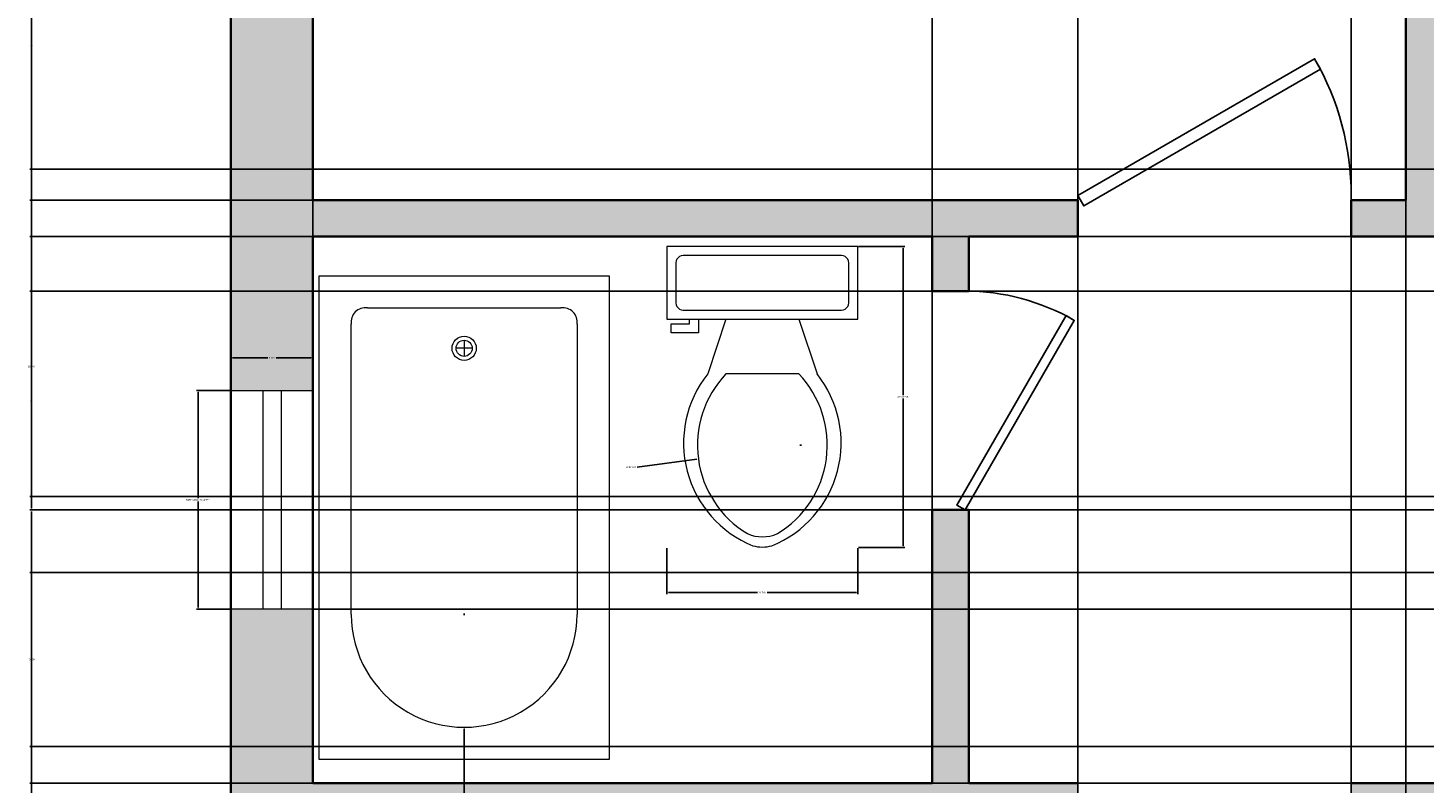
# Model space of a CAD drawing. Units: inches. Extents: x 2800 to 3283, y 1752 to 2114.
# Tile 2 of 6: x 2800 to 2954, y 1903 to 1986. Entities that reach past the tile are written whole.
import ezdxf

# ---------------------------------------------------------------- set-up
doc = ezdxf.new("R2010")
doc.units = ezdxf.units.IN
for name, color, linetype, lineweight in [('A-ANNO-DIMS', 2, 'Continuous', 18), ('A-DOOR', 3, 'Continuous', 25), ('A-FLOR-FIXT', 9, 'Continuous', 18), ('A-GLAZ', 4, 'Continuous', 18), ('A-WALL', 7, 'Continuous', 35)]:
    doc.layers.add(name, color=color, linetype=linetype, lineweight=lineweight)
doc.layers.add('A-WALL-PATT', color=18, linetype='Continuous', lineweight=13, true_color=0x000000)
doc.styles.get("Standard").update_dxf_attribs({"font": 'arial.ttf'})
doc.dimstyles.get("Standard").update_dxf_attribs({"dimtxt": 0.18, "dimasz": 0.18, "dimexe": 0.18, "dimexo": 0.0625, "dimgap": 0.09, "dimtad": 0, "dimtih": 1, "dimtoh": 1, "dimdec": 4, "dimzin": 0, "dimdsep": 46, "dimtxsty": 'Standard', "dimcen": 0.09, "dimadec": 0, "dimazin": 0, "dimtfac": 1, "dimtdec": 4, "dimtofl": 0, "dimtmove": 0, "dimatfit": 3, "dimfxl": 1, "dimtolj": 1, "dimtzin": 0, "dimarcsym": 0})

# ---------------------------------------------------------------- blocks, each defined once
blk = doc.blocks.new('Bath Tub - 26 x 60 in.')
for p, q in [((9, -17), (9, -19)), ((8, -18), (10, -18))]:
    blk.add_line(p, q)
blk.add_lwpolyline([(0, -36), (0, 0), (60, 0), (60, -36)], close=True)
for points in [[(6, -4), (42, -4)], [(4, -30), (4, -6)], [(42, -32), (6, -32)]]:
    blk.add_lwpolyline(points)
for radius in [1.5, 1]:
    blk.add_circle((9, -18), radius)
for centre, radius, start, end in [((5.75, -5.75), 1.77, 81.8699, 188.1301), ((42, -18), 14, 270, 90), ((5.75, -30.25), 1.77, 171.8699, 278.1301)]:
    blk.add_arc(centre, radius, start, end)
blk = doc.blocks.new('Toilet - top')
for p, q in [((9.5, -6), (9.5, -2)), ((-10, -8.5), (-8, -8.5)), ((-10, -9.5), (-10, -8.5)), ((-8, -8.5), (-8, -8)), ((-7, -8), (-7, -9.5)), ((-4, -8), (-6, -14)), ((4, -8), (6, -14)), ((-7, -9.5), (-10, -9.5)), ((4, -14), (-4, -14))]:
    blk.add_line(p, q)
blk.add_lwpolyline([(10.5, -8), (10.5, 0), (-10.5, 0), (-10.5, -8)], close=True)
for points in [[(8.5, -1), (-8.5, -1)], [(-9.5, -2), (-9.5, -6)], [(-8.5, -7), (8.5, -7)]]:
    blk.add_lwpolyline(points)
for centre, radius, start, end in [((-8.62, -1.88), 0.884, 81.8699, 188.1301), ((8.62, -1.88), 0.884, 351.8699, 98.1301), ((-8.62, -6.12), 0.884, 171.8699, 278.1301), ((8.62, -6.12), 0.884, 261.8699, 8.1301), ((3.52, -21.58), 12.17, 141.4691, 247.9714), ((4.2, -21.82), 11.33, 136.3677, 238.9468), ((-3.52, -21.58), 12.17, 292.0284, 38.5307), ((-4.2, -21.82), 11.33, 301.053, 43.6321), ((0, -27.88), 4, 245.7318, 294.2682), ((0, -29), 4, 254.8605, 285.1395)]:
    blk.add_arc(centre, radius, start, end)
blk = doc.blocks.new('*U12')
for p, q in [((0, 0), (0, -6)), ((40, 0), (40, -6))]:
    blk.add_line(p, q)
blk.add_lwpolyline([(0, 0), (34.64, 20), (35.52, 18.48), (0.87, -1.52)], close=True)
blk.add_arc((0, 0), 40, 0, 30)
blk = doc.blocks.new('WIN-24')
for p, q in [((3.5, 24), (3.5, 0)), ((5.5, 24), (5.5, 0))]:
    blk.add_line(p, q)
for points in [[(0, 24), (9, 24)], [(9, 0), (0, 0)]]:
    blk.add_lwpolyline(points)
blk = doc.blocks.new('*D21')
at = {"layer": 'A-ANNO-DIMS', "color": 0, "lineweight": -2, "transparency": 16777216}
for p, q in [((2822.48, 1946.35), (2818.76, 1946.35)), ((2818.94, 1946.17), (2818.94, 1934.54)), ((2818.94, 1922.53), (2818.94, 1934.17)), ((2822.48, 1922.35), (2818.76, 1922.35))]:
    blk.add_line(p, q, dxfattribs=at)
at = {"layer": 'A-ANNO-DIMS', "color": 0, "transparency": 16777216}
for points in [[(2818.91, 1946.17), (2818.97, 1946.17), (2818.94, 1946.35)], [(2818.91, 1922.53), (2818.97, 1922.53), (2818.94, 1922.35)]]:
    blk.add_solid(points, dxfattribs=at)
at = {"layer": 'Defpoints', "color": 0, "transparency": 16777216}
for p in [(2818.94, 1946.35), (2822.54, 1946.35), (2822.54, 1922.35)]:
    blk.add_point(p, dxfattribs=at)
at = {"layer": 'A-ANNO-DIMS', "color": 0, "transparency": 16777216, "insert": (2818.94, 1934.35), "char_height": 0.18, "attachment_point": 5}
blk.add_mtext('\\A1;BATH WINDOW 24 TYP.', dxfattribs=at)
blk = doc.blocks.new('*D22')
at = {"layer": 'A-ANNO-DIMS', "color": 0, "lineweight": -2, "transparency": 16777216}
for p, q in [((2822.54, 1946.42), (2822.54, 1950.13)), ((2822.72, 1949.95), (2826.59, 1949.95)), ((2831.36, 1949.95), (2827.5, 1949.95)), ((2831.54, 1946.42), (2831.54, 1950.13))]:
    blk.add_line(p, q, dxfattribs=at)
at = {"layer": 'A-ANNO-DIMS', "color": 0, "transparency": 16777216}
for points in [[(2822.72, 1949.98), (2822.72, 1949.92), (2822.54, 1949.95)], [(2831.36, 1949.98), (2831.36, 1949.92), (2831.54, 1949.95)]]:
    blk.add_solid(points, dxfattribs=at)
at = {"layer": 'Defpoints', "color": 0, "transparency": 16777216}
for p in [(2831.54, 1949.95), (2822.54, 1946.35), (2831.54, 1946.35)]:
    blk.add_point(p, dxfattribs=at)
at = {"layer": 'A-ANNO-DIMS', "color": 0, "transparency": 16777216, "insert": (2827.04, 1949.95), "char_height": 0.18, "attachment_point": 5}
blk.add_mtext('\\A1;9 TYP.', dxfattribs=at)
blk = doc.blocks.new('*D33')
at = {"layer": 'A-ANNO-DIMS', "color": 0, "lineweight": -2, "transparency": 16777216}
for p, q in [((2891.45, 1962.18), (2896.53, 1962.18)), ((2896.35, 1962), (2896.35, 1945.84)), ((2896.35, 1929.31), (2896.35, 1945.47)), ((2891.45, 1929.13), (2896.53, 1929.13))]:
    blk.add_line(p, q, dxfattribs=at)
at = {"layer": 'A-ANNO-DIMS', "color": 0, "transparency": 16777216}
for points in [[(2896.32, 1962), (2896.38, 1962), (2896.35, 1962.18)], [(2896.32, 1929.31), (2896.38, 1929.31), (2896.35, 1929.13)]]:
    blk.add_solid(points, dxfattribs=at)
at = {"layer": 'Defpoints', "color": 0, "transparency": 16777216}
for p in [(2891.39, 1962.18), (2896.35, 1962.18), (2891.39, 1929.13)]:
    blk.add_point(p, dxfattribs=at)
at = {"layer": 'A-ANNO-DIMS', "color": 0, "transparency": 16777216, "insert": (2896.35, 1945.66), "char_height": 0.18, "attachment_point": 5}
blk.add_mtext('\\A1;WC 33 TYP.', dxfattribs=at)
blk = doc.blocks.new('*D34')
at = {"layer": 'A-ANNO-DIMS', "color": 0, "lineweight": -2, "transparency": 16777216}
for p, q in [((2870.39, 1929.07), (2870.39, 1924)), ((2891.39, 1929.07), (2891.39, 1924)), ((2870.57, 1924.18), (2880.36, 1924.18)), ((2891.21, 1924.18), (2881.42, 1924.18))]:
    blk.add_line(p, q, dxfattribs=at)
at = {"layer": 'A-ANNO-DIMS', "color": 0, "transparency": 16777216}
for points in [[(2870.57, 1924.21), (2870.57, 1924.15), (2870.39, 1924.18)], [(2891.21, 1924.21), (2891.21, 1924.15), (2891.39, 1924.18)]]:
    blk.add_solid(points, dxfattribs=at)
at = {"layer": 'Defpoints', "color": 0, "transparency": 16777216}
for p in [(2870.39, 1929.13), (2891.39, 1929.13), (2891.39, 1924.18)]:
    blk.add_point(p, dxfattribs=at)
at = {"layer": 'A-ANNO-DIMS', "color": 0, "transparency": 16777216, "insert": (2880.89, 1924.18), "char_height": 0.18, "attachment_point": 5}
blk.add_mtext('\\A1;21 TYP.', dxfattribs=at)
blk = doc.blocks.new('*D44')
at = {"layer": 'A-ANNO-DIMS', "color": 0, "lineweight": -2, "transparency": 16777216}
for p, q in [((2822.48, 2092.27), (2800.45, 2092.27)), ((2800.63, 2092.09), (2800.63, 1933.45)), ((2800.63, 1774.45), (2800.63, 1933.09)), ((2822.48, 1774.27), (2800.45, 1774.27))]:
    blk.add_line(p, q, dxfattribs=at)
at = {"layer": 'A-ANNO-DIMS', "color": 0, "transparency": 16777216}
for points in [[(2800.6, 2092.09), (2800.66, 2092.09), (2800.63, 2092.27)], [(2800.6, 1774.45), (2800.66, 1774.45), (2800.63, 1774.27)]]:
    blk.add_solid(points, dxfattribs=at)
at = {"layer": 'Defpoints', "color": 0, "transparency": 16777216}
for p in [(2800.63, 2092.27), (2822.54, 2092.27), (2822.54, 1774.27)]:
    blk.add_point(p, dxfattribs=at)
at = {"layer": 'A-ANNO-DIMS', "color": 0, "transparency": 16777216, "insert": (2800.63, 1933.27), "char_height": 0.18, "attachment_point": 5}
blk.add_mtext('\\A1;318', dxfattribs=at)
blk = doc.blocks.new('*D45')
at = {"layer": 'A-ANNO-DIMS', "color": 0, "lineweight": -2, "transparency": 16777216}
for p, q in [((2831.54, 1967.33), (2831.54, 2114.36)), ((2831.72, 2114.18), (2891.26, 2114.18)), ((2951.36, 2114.18), (2891.82, 2114.18)), ((2951.54, 1967.33), (2951.54, 2114.36))]:
    blk.add_line(p, q, dxfattribs=at)
at = {"layer": 'A-ANNO-DIMS', "color": 0, "transparency": 16777216}
for points in [[(2831.72, 2114.21), (2831.72, 2114.15), (2831.54, 2114.18)], [(2951.36, 2114.21), (2951.36, 2114.15), (2951.54, 2114.18)]]:
    blk.add_solid(points, dxfattribs=at)
at = {"layer": 'Defpoints', "color": 0, "transparency": 16777216}
for p in [(2951.54, 2114.18), (2831.54, 1967.27), (2951.54, 1967.27)]:
    blk.add_point(p, dxfattribs=at)
at = {"layer": 'A-ANNO-DIMS', "color": 0, "transparency": 16777216, "insert": (2891.54, 2114.18), "char_height": 0.18, "attachment_point": 5}
blk.add_mtext('\\A1;120', dxfattribs=at)
blk = doc.blocks.new('*D49')
at = {"layer": 'A-ANNO-DIMS', "color": 0, "lineweight": -2, "transparency": 16777216}
for p, q in [((2831.48, 2083.27), (2800.45, 2083.27)), ((2800.63, 2083.09), (2800.63, 2025.45)), ((2800.63, 1967.45), (2800.63, 2025.09)), ((2831.48, 1967.27), (2800.45, 1967.27))]:
    blk.add_line(p, q, dxfattribs=at)
at = {"layer": 'A-ANNO-DIMS', "color": 0, "transparency": 16777216}
for points in [[(2800.6, 2083.09), (2800.66, 2083.09), (2800.63, 2083.27)], [(2800.6, 1967.45), (2800.66, 1967.45), (2800.63, 1967.27)]]:
    blk.add_solid(points, dxfattribs=at)
at = {"layer": 'Defpoints', "color": 0, "transparency": 16777216}
for p in [(2800.63, 2083.27), (2831.54, 2083.27), (2831.54, 1967.27)]:
    blk.add_point(p, dxfattribs=at)
at = {"layer": 'A-ANNO-DIMS', "color": 0, "transparency": 16777216, "insert": (2800.63, 2025.27), "char_height": 0.18, "attachment_point": 5}
blk.add_mtext('\\A1;116', dxfattribs=at)
blk = doc.blocks.new('*D50')
at = {"layer": 'A-ANNO-DIMS', "color": 0, "lineweight": -2, "transparency": 16777216}
for p, q in [((2831.48, 1963.27), (2800.45, 1963.27)), ((2800.63, 1963.09), (2800.63, 1933.45)), ((2800.63, 1903.45), (2800.63, 1933.09)), ((2831.48, 1903.27), (2800.45, 1903.27))]:
    blk.add_line(p, q, dxfattribs=at)
at = {"layer": 'A-ANNO-DIMS', "color": 0, "transparency": 16777216}
for points in [[(2800.6, 1963.09), (2800.66, 1963.09), (2800.63, 1963.27)], [(2800.6, 1903.45), (2800.66, 1903.45), (2800.63, 1903.27)]]:
    blk.add_solid(points, dxfattribs=at)
at = {"layer": 'Defpoints', "color": 0, "transparency": 16777216}
for p in [(2800.63, 1963.27), (2831.54, 1963.27), (2831.54, 1903.27)]:
    blk.add_point(p, dxfattribs=at)
at = {"layer": 'A-ANNO-DIMS', "color": 0, "transparency": 16777216, "insert": (2800.63, 1933.27), "char_height": 0.18, "attachment_point": 5}
blk.add_mtext('\\A1;60', dxfattribs=at)
blk = doc.blocks.new('*D54')
at = {"layer": 'A-ANNO-DIMS', "color": 0, "lineweight": -2, "transparency": 16777216}
for p, q in [((2831.54, 1903.33), (2831.54, 2114.36)), ((2831.72, 2114.18), (2865.32, 2114.18)), ((2899.36, 2114.18), (2865.76, 2114.18)), ((2899.54, 1903.33), (2899.54, 2114.36))]:
    blk.add_line(p, q, dxfattribs=at)
at = {"layer": 'A-ANNO-DIMS', "color": 0, "transparency": 16777216}
for points in [[(2831.72, 2114.21), (2831.72, 2114.15), (2831.54, 2114.18)], [(2899.36, 2114.21), (2899.36, 2114.15), (2899.54, 2114.18)]]:
    blk.add_solid(points, dxfattribs=at)
at = {"layer": 'Defpoints', "color": 0, "transparency": 16777216}
for p in [(2899.54, 2114.18), (2831.54, 1903.27), (2899.54, 1903.27)]:
    blk.add_point(p, dxfattribs=at)
at = {"layer": 'A-ANNO-DIMS', "color": 0, "transparency": 16777216, "insert": (2865.54, 2114.18), "char_height": 0.18, "attachment_point": 5}
blk.add_mtext('\\A1;68', dxfattribs=at)
blk = doc.blocks.new('*D64')
at = {"layer": 'A-ANNO-DIMS', "color": 0, "lineweight": -2, "transparency": 16777216}
for p, q in [((2831.61, 1922.35), (3282.64, 1922.35)), ((3282.46, 1922.17), (3282.46, 1912.99)), ((3282.46, 1903.45), (3282.46, 1912.63)), ((2831.61, 1903.27), (3282.64, 1903.27))]:
    blk.add_line(p, q, dxfattribs=at)
at = {"layer": 'A-ANNO-DIMS', "color": 0, "transparency": 16777216}
for points in [[(3282.43, 1922.17), (3282.49, 1922.17), (3282.46, 1922.35)], [(3282.43, 1903.45), (3282.49, 1903.45), (3282.46, 1903.27)]]:
    blk.add_solid(points, dxfattribs=at)
at = {"layer": 'Defpoints', "color": 0, "transparency": 16777216}
for p in [(2831.54, 1922.35), (3282.46, 1922.35), (2831.54, 1903.27)]:
    blk.add_point(p, dxfattribs=at)
at = {"layer": 'A-ANNO-DIMS', "color": 0, "transparency": 16777216, "insert": (3282.46, 1912.81), "char_height": 0.18, "attachment_point": 5}
blk.add_mtext('\\A1;19.085', dxfattribs=at)
blk = doc.blocks.new('*D65')
at = {"layer": 'A-ANNO-DIMS', "color": 0, "lineweight": -2, "transparency": 16777216}
for p, q in [((3251.48, 1926.4), (2800.45, 1926.4)), ((2800.63, 1926.22), (2800.63, 1917.02)), ((2800.63, 1907.45), (2800.63, 1916.65)), ((3251.48, 1907.27), (2800.45, 1907.27))]:
    blk.add_line(p, q, dxfattribs=at)
at = {"layer": 'A-ANNO-DIMS', "color": 0, "transparency": 16777216}
for points in [[(2800.6, 1926.22), (2800.66, 1926.22), (2800.63, 1926.4)], [(2800.6, 1907.45), (2800.66, 1907.45), (2800.63, 1907.27)]]:
    blk.add_solid(points, dxfattribs=at)
at = {"layer": 'Defpoints', "color": 0, "transparency": 16777216}
for p in [(2800.63, 1926.4), (3251.54, 1926.4), (3251.54, 1907.27)]:
    blk.add_point(p, dxfattribs=at)
at = {"layer": 'A-ANNO-DIMS', "color": 0, "transparency": 16777216, "insert": (2800.63, 1916.83), "char_height": 0.18, "attachment_point": 5}
blk.add_mtext('\\A1;19.128', dxfattribs=at)
blk = doc.blocks.new('*D66')
at = {"layer": 'A-ANNO-DIMS', "color": 0, "lineweight": -2, "transparency": 16777216}
for p, q in [((2915.54, 1899.33), (2915.54, 2114.36)), ((2915.72, 2114.18), (2930.32, 2114.18)), ((2945.36, 2114.18), (2930.76, 2114.18)), ((2945.54, 1899.33), (2945.54, 2114.36))]:
    blk.add_line(p, q, dxfattribs=at)
at = {"layer": 'A-ANNO-DIMS', "color": 0, "transparency": 16777216}
for points in [[(2915.72, 2114.21), (2915.72, 2114.15), (2915.54, 2114.18)], [(2945.36, 2114.21), (2945.36, 2114.15), (2945.54, 2114.18)]]:
    blk.add_solid(points, dxfattribs=at)
at = {"layer": 'Defpoints', "color": 0, "transparency": 16777216}
for p in [(2945.54, 2114.18), (2915.54, 1899.27), (2945.54, 1899.27)]:
    blk.add_point(p, dxfattribs=at)
at = {"layer": 'A-ANNO-DIMS', "color": 0, "transparency": 16777216, "insert": (2930.54, 2114.18), "char_height": 0.18, "attachment_point": 5}
blk.add_mtext('\\A1;30', dxfattribs=at)
blk = doc.blocks.new('*D67')
at = {"layer": 'A-ANNO-DIMS', "color": 0, "lineweight": -2, "transparency": 16777216}
for p, q in [((2945.54, 1899.33), (2945.54, 2114.36)), ((2945.72, 2114.18), (2948.39, 2114.18)), ((2951.36, 2114.18), (2948.69, 2114.18)), ((2951.54, 1899.33), (2951.54, 2114.36))]:
    blk.add_line(p, q, dxfattribs=at)
at = {"layer": 'A-ANNO-DIMS', "color": 0, "transparency": 16777216}
for points in [[(2945.72, 2114.21), (2945.72, 2114.15), (2945.54, 2114.18)], [(2951.36, 2114.21), (2951.36, 2114.15), (2951.54, 2114.18)]]:
    blk.add_solid(points, dxfattribs=at)
at = {"layer": 'Defpoints', "color": 0, "transparency": 16777216}
for p in [(2951.54, 2114.18), (2945.54, 1899.27), (2951.54, 1899.27)]:
    blk.add_point(p, dxfattribs=at)
at = {"layer": 'A-ANNO-DIMS', "color": 0, "transparency": 16777216, "insert": (2948.54, 2114.18), "char_height": 0.18, "attachment_point": 5}
blk.add_mtext('\\A1;6', dxfattribs=at)
blk = doc.blocks.new('*D68')
at = {"layer": 'A-ANNO-DIMS', "color": 0, "lineweight": -2, "transparency": 16777216}
for p, q in [((3175.48, 1957.27), (2800.45, 1957.27)), ((2800.63, 1957.09), (2800.63, 1945.45)), ((2800.63, 1933.45), (2800.63, 1945.09)), ((3175.48, 1933.27), (2800.45, 1933.27))]:
    blk.add_line(p, q, dxfattribs=at)
at = {"layer": 'A-ANNO-DIMS', "color": 0, "transparency": 16777216}
for points in [[(2800.6, 1957.09), (2800.66, 1957.09), (2800.63, 1957.27)], [(2800.6, 1933.45), (2800.66, 1933.45), (2800.63, 1933.27)]]:
    blk.add_solid(points, dxfattribs=at)
at = {"layer": 'Defpoints', "color": 0, "transparency": 16777216}
for p in [(2800.63, 1957.27), (3175.54, 1957.27), (3175.54, 1933.27)]:
    blk.add_point(p, dxfattribs=at)
at = {"layer": 'A-ANNO-DIMS', "color": 0, "transparency": 16777216, "insert": (2800.63, 1945.27), "char_height": 0.18, "attachment_point": 5}
blk.add_mtext('\\A1;24', dxfattribs=at)
blk = doc.blocks.new('*D69')
at = {"layer": 'A-ANNO-DIMS', "color": 0, "lineweight": -2, "transparency": 16777216}
for p, q in [((3175.48, 1963.27), (2800.45, 1963.27)), ((2800.63, 1963.09), (2800.63, 1960.45)), ((2800.63, 1957.45), (2800.63, 1960.09)), ((3175.48, 1957.27), (2800.45, 1957.27))]:
    blk.add_line(p, q, dxfattribs=at)
at = {"layer": 'A-ANNO-DIMS', "color": 0, "transparency": 16777216}
for points in [[(2800.6, 1963.09), (2800.66, 1963.09), (2800.63, 1963.27)], [(2800.6, 1957.45), (2800.66, 1957.45), (2800.63, 1957.27)]]:
    blk.add_solid(points, dxfattribs=at)
at = {"layer": 'Defpoints', "color": 0, "transparency": 16777216}
for p in [(2800.63, 1963.27), (3175.54, 1963.27), (3175.54, 1957.27)]:
    blk.add_point(p, dxfattribs=at)
at = {"layer": 'A-ANNO-DIMS', "color": 0, "transparency": 16777216, "insert": (2800.63, 1960.27), "char_height": 0.18, "attachment_point": 5}
blk.add_mtext('\\A1;6', dxfattribs=at)
blk = doc.blocks.new('*D71')
at = {"layer": 'A-ANNO-DIMS', "color": 0, "lineweight": -2, "transparency": 16777216}
for p, q in [((3037.48, 1903.27), (2800.45, 1903.27)), ((2800.63, 1903.09), (2800.63, 1879.54)), ((2800.63, 1855.63), (2800.63, 1879.18)), ((3037.48, 1855.45), (2800.45, 1855.45))]:
    blk.add_line(p, q, dxfattribs=at)
at = {"layer": 'A-ANNO-DIMS', "color": 0, "transparency": 16777216}
for points in [[(2800.6, 1903.09), (2800.66, 1903.09), (2800.63, 1903.27)], [(2800.6, 1855.63), (2800.66, 1855.63), (2800.63, 1855.45)]]:
    blk.add_solid(points, dxfattribs=at)
at = {"layer": 'Defpoints', "color": 0, "transparency": 16777216}
for p in [(2800.63, 1903.27), (3037.54, 1903.27), (3037.54, 1855.45)]:
    blk.add_point(p, dxfattribs=at)
at = {"layer": 'A-ANNO-DIMS', "color": 0, "transparency": 16777216, "insert": (2800.63, 1879.36), "char_height": 0.18, "attachment_point": 5}
blk.add_mtext('\\A1;47.82', dxfattribs=at)
blk = doc.blocks.new('*D76')
at = {"layer": 'A-ANNO-DIMS', "color": 0, "lineweight": -2, "transparency": 16777216}
for p, q in [((3095.48, 1903.27), (2800.45, 1903.27)), ((2800.63, 1903.09), (2800.63, 1891.49)), ((2800.63, 1879.52), (2800.63, 1891.12)), ((3103.48, 1879.34), (2800.45, 1879.34))]:
    blk.add_line(p, q, dxfattribs=at)
at = {"layer": 'A-ANNO-DIMS', "color": 0, "transparency": 16777216}
for points in [[(2800.6, 1903.09), (2800.66, 1903.09), (2800.63, 1903.27)], [(2800.6, 1879.52), (2800.66, 1879.52), (2800.63, 1879.34)]]:
    blk.add_solid(points, dxfattribs=at)
at = {"layer": 'Defpoints', "color": 0, "transparency": 16777216}
for p in [(3095.54, 1903.27), (2800.63, 1879.34), (3103.54, 1879.34)]:
    blk.add_point(p, dxfattribs=at)
at = {"layer": 'A-ANNO-DIMS', "color": 0, "transparency": 16777216, "insert": (2800.63, 1891.31), "char_height": 0.18, "attachment_point": 5}
blk.add_mtext('\\A1;23.93', dxfattribs=at)
blk = doc.blocks.new('*D77')
at = {"layer": 'A-ANNO-DIMS', "color": 0, "lineweight": -2, "transparency": 16777216}
for p, q in [((3076.62, 2072.66), (2800.45, 2072.66)), ((2800.63, 2072.48), (2800.63, 2021.84)), ((2800.63, 1970.84), (2800.63, 2021.48)), ((3076.62, 1970.66), (2800.45, 1970.66))]:
    blk.add_line(p, q, dxfattribs=at)
at = {"layer": 'A-ANNO-DIMS', "color": 0, "transparency": 16777216}
for points in [[(2800.6, 2072.48), (2800.66, 2072.48), (2800.63, 2072.66)], [(2800.6, 1970.84), (2800.66, 1970.84), (2800.63, 1970.66)]]:
    blk.add_solid(points, dxfattribs=at)
at = {"layer": 'Defpoints', "color": 0, "transparency": 16777216}
for p in [(3076.68, 2072.66), (2800.63, 1970.66), (3076.68, 1970.66)]:
    blk.add_point(p, dxfattribs=at)
at = {"layer": 'A-ANNO-DIMS', "color": 0, "transparency": 16777216, "insert": (2800.63, 2021.66), "char_height": 0.18, "attachment_point": 5}
blk.add_mtext('\\A1;102', dxfattribs=at)
blk = doc.blocks.new('*D81')
at = {"layer": 'A-ANNO-DIMS', "color": 0, "lineweight": -2, "transparency": 16777216}
for p, q in [((2909.16, 2001.27), (2800.45, 2001.27)), ((2800.63, 2001.09), (2800.63, 1984.45)), ((2800.63, 1967.45), (2800.63, 1984.09)), ((2915.48, 1967.27), (2800.45, 1967.27))]:
    blk.add_line(p, q, dxfattribs=at)
at = {"layer": 'A-ANNO-DIMS', "color": 0, "transparency": 16777216}
for points in [[(2800.6, 2001.09), (2800.66, 2001.09), (2800.63, 2001.27)], [(2800.6, 1967.45), (2800.66, 1967.45), (2800.63, 1967.27)]]:
    blk.add_solid(points, dxfattribs=at)
at = {"layer": 'Defpoints', "color": 0, "transparency": 16777216}
for p in [(2800.63, 2001.27), (2909.23, 2001.27), (2915.54, 1967.27)]:
    blk.add_point(p, dxfattribs=at)
at = {"layer": 'A-ANNO-DIMS', "color": 0, "transparency": 16777216, "insert": (2800.63, 1984.27), "char_height": 0.18, "attachment_point": 5}
blk.add_mtext('\\A1;34', dxfattribs=at)
blk = doc.blocks.new('*D86')
at = {"layer": 'A-ANNO-DIMS', "color": 0, "lineweight": -2, "transparency": 16777216}
for p, q in [((2955.48, 1963.27), (2800.45, 1963.27)), ((2800.63, 1963.09), (2800.63, 1949.18)), ((2800.63, 1934.9), (2800.63, 1948.81)), ((3008.9, 1934.72), (2800.45, 1934.72))]:
    blk.add_line(p, q, dxfattribs=at)
at = {"layer": 'A-ANNO-DIMS', "color": 0, "transparency": 16777216}
for points in [[(2800.6, 1963.09), (2800.66, 1963.09), (2800.63, 1963.27)], [(2800.6, 1934.9), (2800.66, 1934.9), (2800.63, 1934.72)]]:
    blk.add_solid(points, dxfattribs=at)
at = {"layer": 'Defpoints', "color": 0, "transparency": 16777216}
for p in [(2955.54, 1963.27), (2800.63, 1934.72), (3008.97, 1934.72)]:
    blk.add_point(p, dxfattribs=at)
at = {"layer": 'A-ANNO-DIMS', "color": 0, "transparency": 16777216, "insert": (2800.63, 1949), "char_height": 0.18, "attachment_point": 5}
blk.add_mtext('\\A1;28.547', dxfattribs=at)
blk = doc.blocks.new('*D87')
at = {"layer": 'A-ANNO-DIMS', "color": 0, "lineweight": -2, "transparency": 16777216}
for p, q in [((2848.06, 1921.79), (2848.24, 1921.79)), ((2848.15, 1921.7), (2848.15, 1921.88)), ((2848.15, 1901.96), (2848.15, 1909.22)), ((2848.33, 1901.96), (2848.15, 1901.96))]:
    blk.add_line(p, q, dxfattribs=at)
at = {"layer": 'A-ANNO-DIMS', "color": 0, "transparency": 16777216}
blk.add_solid([(2848.18, 1909.22), (2848.12, 1909.22), (2848.15, 1909.4)], dxfattribs=at)
at = {"layer": 'Defpoints', "color": 0, "transparency": 16777216}
for p in [(2848.15, 1921.79), (2848.15, 1909.4)]:
    blk.add_point(p, dxfattribs=at)
at = {"layer": 'A-ANNO-DIMS', "color": 0, "transparency": 16777216, "insert": (2849.06, 1901.96), "char_height": 0.18, "attachment_point": 5}
blk.add_mtext('\\A1;2X R12.391', dxfattribs=at)
blk = doc.blocks.new('*D89')
at = {"layer": 'A-ANNO-DIMS', "color": 0, "lineweight": -2, "transparency": 16777216}
for p, q in [((2885, 1940.36), (2885.18, 1940.36)), ((2885.09, 1940.27), (2885.09, 1940.45)), ((2867.13, 1937.94), (2873.68, 1938.83))]:
    blk.add_line(p, q, dxfattribs=at)
at = {"layer": 'A-ANNO-DIMS', "color": 0, "transparency": 16777216}
blk.add_solid([(2873.68, 1938.86), (2873.69, 1938.8), (2873.86, 1938.85)], dxfattribs=at)
at = {"layer": 'Defpoints', "color": 0, "transparency": 16777216}
for p in [(2885.09, 1940.36), (2873.86, 1938.85)]:
    blk.add_point(p, dxfattribs=at)
at = {"layer": 'A-ANNO-DIMS', "color": 0, "transparency": 16777216, "insert": (2866.45, 1937.94), "char_height": 0.18, "attachment_point": 5}
blk.add_mtext('\\A1;4X R11.33', dxfattribs=at)

msp = doc.modelspace()

# ---------------------------------------------------------------- hatches: boundary and pattern name
at = {"layer": 'A-WALL-PATT'}
h = msp.add_hatch(color=256, dxfattribs=at)
h.dxf.hatch_style = 1
h.paths.add_polyline_path([(2868.6629, 2092.2695), (2822.5432, 2092.2695), (2822.5432, 1946.3547), (2831.5432, 1946.3547), (2831.5432, 1963.2695), (2899.5432, 1963.2695), (2899.5432, 1957.2695), (2903.5432, 1957.2695), (2903.5432, 1963.2695), (2915.5432, 1963.2695), (2915.5432, 1967.2695), (2831.5432, 1967.2695), (2831.5432, 2083.2695), (2868.6629, 2083.2695)])
h = msp.add_hatch(color=256, dxfattribs=at)
h.dxf.hatch_style = 1
h.paths.add_polyline_path([(3023.883, 2092.2695), (2916.6629, 2092.2695), (2916.6629, 2083.2695), (2951.5432, 2083.2695), (2951.5432, 2011.2695), (2951.5432, 1967.2695), (2945.5432, 1967.2695), (2945.5432, 1963.2695), (2955.5432, 1963.2695), (2955.5432, 2083.2695), (3023.883, 2083.2695)])
h = msp.add_hatch(color=256, dxfattribs=at)
h.dxf.hatch_style = 1
h.paths.add_polyline_path([(2863.5307, 1783.2695), (2831.5432, 1783.2695), (2831.5432, 1899.2695), (2903.5432, 1899.2695), (2915.5432, 1899.2695), (2915.5432, 1903.2695), (2903.5432, 1903.2695), (2903.5432, 1933.2695), (2899.5432, 1933.2695), (2899.5432, 1903.2695), (2831.5432, 1903.2695), (2831.5432, 1922.3547), (2822.5432, 1922.3547), (2822.5432, 1774.2695), (2863.5307, 1774.2695)])
h = msp.add_hatch(color=256, dxfattribs=at)
h.dxf.hatch_style = 1
h.paths.add_polyline_path([(2967.5432, 1783.2695), (2955.5432, 1783.2695), (2955.5432, 1903.2695), (2945.5432, 1903.2695), (2945.5432, 1899.2695), (2951.5432, 1899.2695), (2951.5432, 1783.2695), (2911.5307, 1783.2695), (2911.5307, 1774.2695), (2967.5432, 1774.2695)])

# ---------------------------------------------------------------- linework, layer by layer
at = {"layer": 'A-WALL'}
for p, q in [((2831.5432, 1967.2695), (2831.5432, 2083.2695)), ((2951.5432, 1967.2695), (2951.5432, 2083.2695)), ((2831.5432, 1967.2695), (2915.5432, 1967.2695)), ((2915.5432, 1967.2695), (2915.5432, 1963.2695)), ((2945.5432, 1967.2695), (2945.5432, 1963.2695)), ((2945.5432, 1967.2695), (2951.5432, 1967.2695)), ((2831.5432, 1963.2695), (2899.5432, 1963.2695)), ((2831.5432, 1903.2695), (2831.5432, 1963.2695)), ((2899.5432, 1957.2695), (2899.5432, 1963.2695)), ((2903.5432, 1963.2695), (2915.5432, 1963.2695)), ((2903.5432, 1957.2695), (2903.5432, 1963.2695)), ((2945.5432, 1963.2695), (2955.5432, 1963.2695)), ((2899.5432, 1957.2695), (2903.5432, 1957.2695)), ((2899.5432, 1903.2695), (2899.5432, 1933.2695)), ((2899.5432, 1933.2695), (2903.5432, 1933.2695)), ((2903.5432, 1903.2695), (2903.5432, 1933.2695)), ((2899.5432, 1903.2695), (2831.5432, 1903.2695)), ((2915.5432, 1903.2695), (2903.5432, 1903.2695)), ((2955.5432, 1903.2695), (2945.5432, 1903.2695))]:
    msp.add_line(p, q, dxfattribs=at)
msp.add_lwpolyline([(2967.5432, 1774.2695), (2822.5432, 1774.2695), (2822.5432, 2092.2695), (3260.5432, 2092.2695), (3260.5432, 1774.2695), (3015.5432, 1774.2695)], dxfattribs=at)

# ---------------------------------------------------------------- block references
at = {"layer": 'A-DOOR', "xscale": 0.75, "yscale": 0.75, "zscale": 0.75}
msp.add_blockref('*U12', (2915.5432, 1967.7695), dxfattribs=at)
at = {"layer": 'A-DOOR', "xscale": -0.6, "yscale": 0.6, "zscale": 0.6, "rotation": 270}
msp.add_blockref('*U12', (2903.1432, 1933.2695), dxfattribs=at)
at = {"layer": 'A-FLOR-FIXT'}
msp.add_blockref('Toilet - top', (2880.8908, 1962.1784), dxfattribs=at)
at = {"layer": 'A-FLOR-FIXT', "xscale": 0.8850894228967868, "yscale": 0.8850894228967868, "zscale": 0.8850894228967868, "rotation": 270}
msp.add_blockref('Bath Tub - 26 x 60 in.', (2864.0811, 1958.96), dxfattribs=at)
at = {"layer": 'A-GLAZ'}
msp.add_blockref('WIN-24', (2822.543, 1922.355), dxfattribs=at)

# ---------------------------------------------------------------- dimensions: what is measured, and where the dimension line sits
at = {"layer": 'A-ANNO-DIMS'}
for base, p1, p2, picture, middle in [((2951.5432, 2114.1845), (2831.5432, 1967.2695), (2951.5432, 1967.2695), '*D45', (2891.5432, 2114.1845)), ((2899.5432, 2114.1845), (2831.5432, 1903.2695), (2899.5432, 1903.2695), '*D54', (2865.5432, 2114.1845)), ((2945.5432, 2114.1845), (2915.5432, 1899.2695), (2945.5432, 1899.2695), '*D66', (2930.5432, 2114.1845)), ((2951.5432, 2114.1845), (2945.5432, 1899.2695), (2951.5432, 1899.2695), '*D67', (2948.5432, 2114.1845))]:
    dim = msp.add_linear_dim(base=base, p1=p1, p2=p2, dimstyle='Standard', override={"dimdec": 0, "dimlfac": 1, "dimrnd": 0, "dimzin": 0, "dimdsep": 46, "dimlunit": 2}, dxfattribs=at)
    dim.commit()
    dim.dimension.update_dxf_attribs({"geometry": picture, "text_midpoint": middle})
for base, p1, p2, override, picture, middle in [((2800.6282, 2092.2695), (2822.5432, 1774.2695), (2822.5432, 2092.2695), {"dimdec": 0, "dimlfac": 1, "dimrnd": 0, "dimzin": 0, "dimdsep": 46, "dimlunit": 2}, '*D44', (2800.6282, 1933.2695)), ((2800.6282, 2083.2695), (2831.5432, 1967.2695), (2831.5432, 2083.2695), {"dimdec": 0, "dimlfac": 1, "dimrnd": 0, "dimzin": 0, "dimdsep": 46, "dimlunit": 2}, '*D49', (2800.6282, 2025.2695)), ((2800.6282, 1970.661), (3076.6778, 2072.661), (3076.6778, 1970.661), {"dimdec": 0, "dimlfac": 1, "dimrnd": 0, "dimzin": 0, "dimdsep": 46, "dimlunit": 2}, '*D77', (2800.6282, 2021.661)), ((2800.6282, 2001.2722), (2915.5432, 1967.2695), (2909.2258, 2001.2722), {"dimdec": 0, "dimlfac": 1, "dimrnd": 0, "dimzin": 0, "dimdsep": 46, "dimlunit": 2}, '*D81', (2800.6282, 1984.2708)), ((2800.6282, 1934.7224), (2955.5432, 1963.2695), (3008.9659, 1934.7224), {"dimdec": 3, "dimlfac": 1, "dimrnd": 0, "dimzin": 0, "dimdsep": 46, "dimlunit": 2}, '*D86', (2800.6282, 1948.9959)), ((2800.6282, 1963.2695), (2831.5432, 1903.2695), (2831.5432, 1963.2695), {"dimdec": 0, "dimlfac": 1, "dimrnd": 0, "dimzin": 0, "dimdsep": 46, "dimlunit": 2}, '*D50', (2800.6282, 1933.2695)), ((2800.6282, 1963.2695), (3175.5432, 1957.2695), (3175.5432, 1963.2695), {"dimdec": 0, "dimlfac": 1, "dimrnd": 0, "dimzin": 0, "dimdsep": 46, "dimlunit": 2}, '*D69', (2800.6282, 1960.2695)), ((2800.6282, 1957.2695), (3175.5432, 1933.2695), (3175.5432, 1957.2695), {"dimdec": 0, "dimlfac": 1, "dimrnd": 0, "dimzin": 0, "dimdsep": 46, "dimlunit": 2}, '*D68', (2800.6282, 1945.2695)), ((2800.6282, 1926.3971), (3251.5432, 1907.2695), (3251.5432, 1926.3971), {"dimdec": 3, "dimlfac": 1, "dimrnd": 0, "dimzin": 0, "dimdsep": 46, "dimlunit": 2}, '*D65', (2800.6282, 1916.8333)), ((3282.4582, 1922.3547), (2831.5432, 1903.2695), (2831.5432, 1922.3547), {"dimdec": 3, "dimlfac": 1, "dimrnd": 0, "dimzin": 0, "dimdsep": 46, "dimlunit": 2}, '*D64', (3282.4582, 1912.8121)), ((2800.6282, 1903.2695), (3037.5432, 1855.4517), (3037.5432, 1903.2695), {"dimdec": 2, "dimlfac": 1, "dimrnd": 0, "dimzin": 0, "dimdsep": 46, "dimlunit": 2}, '*D71', (2800.6282, 1879.3606)), ((2800.6282, 1879.3408), (3095.5432, 1903.2695), (3103.5432, 1879.3408), {"dimdec": 2, "dimlfac": 1, "dimrnd": 0, "dimzin": 0, "dimdsep": 46, "dimlunit": 2}, '*D76', (2800.6282, 1891.3052))]:
    dim = msp.add_linear_dim(base=base, p1=p1, p2=p2, angle=90, dimstyle='Standard', override=override, dxfattribs=at)
    dim.commit()
    dim.dimension.update_dxf_attribs({"geometry": picture, "text_midpoint": middle})
for base, p1, p2, text, picture, middle in [((2896.3478, 1962.1784), (2891.3908, 1929.1322), (2891.3908, 1962.1784), 'WC <> TYP.', '*D33', (2896.3478, 1945.6553)), ((2818.9432, 1946.3547), (2822.5432, 1922.3547), (2822.5432, 1946.3547), 'BATH WINDOW <> TYP.', '*D21', (2818.9432, 1934.3547))]:
    dim = msp.add_linear_dim(base=base, p1=p1, p2=p2, angle=90, text=text, dimstyle='Standard', override={"dimdec": 0, "dimlfac": 1, "dimrnd": 0, "dimzin": 0, "dimdsep": 46, "dimlunit": 2}, dxfattribs=at)
    dim.commit()
    dim.dimension.update_dxf_attribs({"geometry": picture, "text_midpoint": middle})
for base, p1, p2, picture, middle in [((2831.5432, 1949.9547), (2822.5432, 1946.3547), (2831.5432, 1946.3547), '*D22', (2827.0432, 1949.9547)), ((2891.3908, 1924.1752), (2870.3908, 1929.1322), (2891.3908, 1929.1322), '*D34', (2880.8908, 1924.1752))]:
    dim = msp.add_linear_dim(base=base, p1=p1, p2=p2, text='<> TYP.', dimstyle='Standard', override={"dimdec": 0, "dimlfac": 1, "dimrnd": 0, "dimzin": 0, "dimdsep": 46, "dimlunit": 2}, dxfattribs=at)
    dim.commit()
    dim.dimension.update_dxf_attribs({"geometry": picture, "text_midpoint": middle})
for center, mpoint, text, override, picture, middle in [((2885.0908, 1940.361), (2873.8627, 1938.851), '4X <>', {"dimdec": 2, "dimlfac": 1, "dimrnd": 0, "dimzin": 0, "dimdsep": 46, "dimlunit": 2}, '*D89', (2867.1258, 1937.9449)), ((2848.1495, 1921.7863), (2848.15, 1909.395), '2X <>', {"dimdec": 3, "dimlfac": 1, "dimrnd": 0, "dimzin": 0, "dimdsep": 46, "dimlunit": 2}, '*D87', (2849.0576, 1901.9603))]:
    dim = msp.add_radius_dim(center=center, mpoint=mpoint, text=text, dimstyle='Standard', override=override, dxfattribs=at)
    dim.commit()
    dim.dimension.update_dxf_attribs({"geometry": picture, "text_midpoint": middle, "dimtype": 164})

doc.saveas('drawing.dxf')
